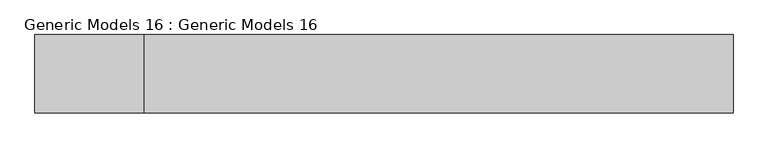
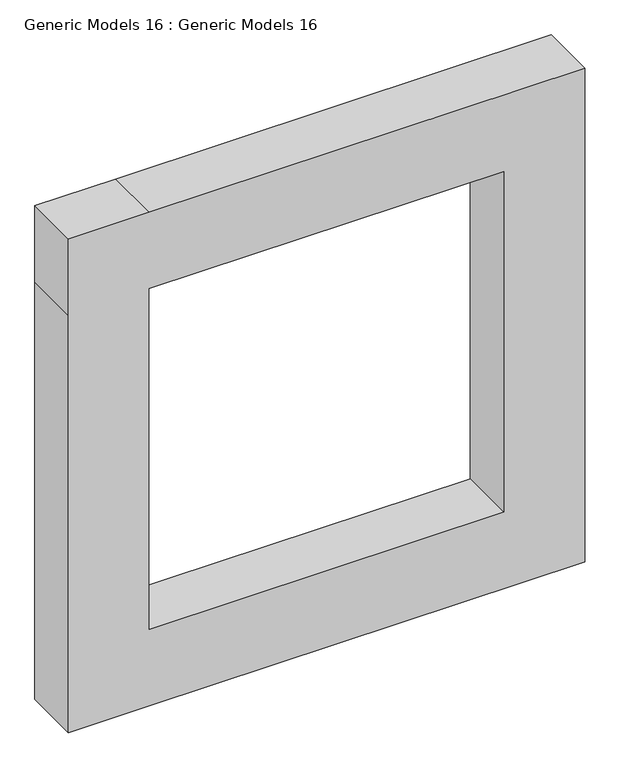
"""IFC4 building model written with IfcOpenShell, lengths in millimetres: proxy geometry, Generic Models 16 : Generic Models 16."""

from ifc_helpers import new_model, si_unit, frame, origin, place, context, project, spatial, polyline, outline, extrude, source, transform, mapped, element, save


def generic_models_16_generic_models_16_6386461c(model_context):
    return source(origin(), model_context, "Body", "SweptSolid", [
        extrude(outline(polyline([(2333.6676291, -5718.4036806), (2495.55, -5718.4036806), (2495.55, -7356.7036806), (2495.55, -7661.5036806), (2190.75, -7661.5036806), (530.2676291, -7661.5036806), (530.2676291, -7356.7036806), (530.2676291, -5718.4036806), (835.0676291, -5718.4036806), (2333.6676291, -5718.4036806)]), holes=[polyline([(835.0676291, -6023.2036806), (835.0676291, -7356.7036806), (2190.75, -7356.7036806), (2190.75, -6023.2036806), (835.0676291, -6023.2036806)])]), frame((0.0, -5690.0708764, 0.0), z_axis=(0.0, 1.0, 0.0), x_axis=(0.0, 0.0, 1.0)), (0.0, 0.0, 1.0), 218.3435662),
    ])


if __name__ == "__main__":
    model = new_model("IFC4")
    model_context = context("Model", 3, world=origin())
    ifc_project = project(units=[si_unit("LENGTHUNIT", "METRE", prefix="MILLI")], contexts=[model_context])
    site = spatial("IfcSite", under=ifc_project)
    building = spatial("IfcBuilding", under=site)
    placement = place(None, origin())
    generic_models_16_generic_models_16_shape = generic_models_16_generic_models_16_6386461c(model_context)
    element("IfcBuildingElementProxy", 1, Name="Generic Models 16 : Generic Models 16", ObjectType="Generic Models 16 : Generic Models 16", at=placement, inside=building, context=model_context, shape_type="MappedRepresentation", body=[
        mapped(generic_models_16_generic_models_16_shape, transform((0.0, 0.0, 0.0), x_axis=(1.0, 0.0, 0.0), y_axis=(0.0, 1.0, 0.0), z_axis=(0.0, 0.0, 1.0))),
    ])
    save(model, "model.ifc")

# Revit data of these elements
# Element 1 (IfcBuildingElementProxy, "Generic Models 16 : Generic Models 16")
#   Materials on its faces: "exterior wall"
# Materials
#   "exterior wall": class "Generic", colour RGB 215 217 121, transparency 0, Cost = 0
